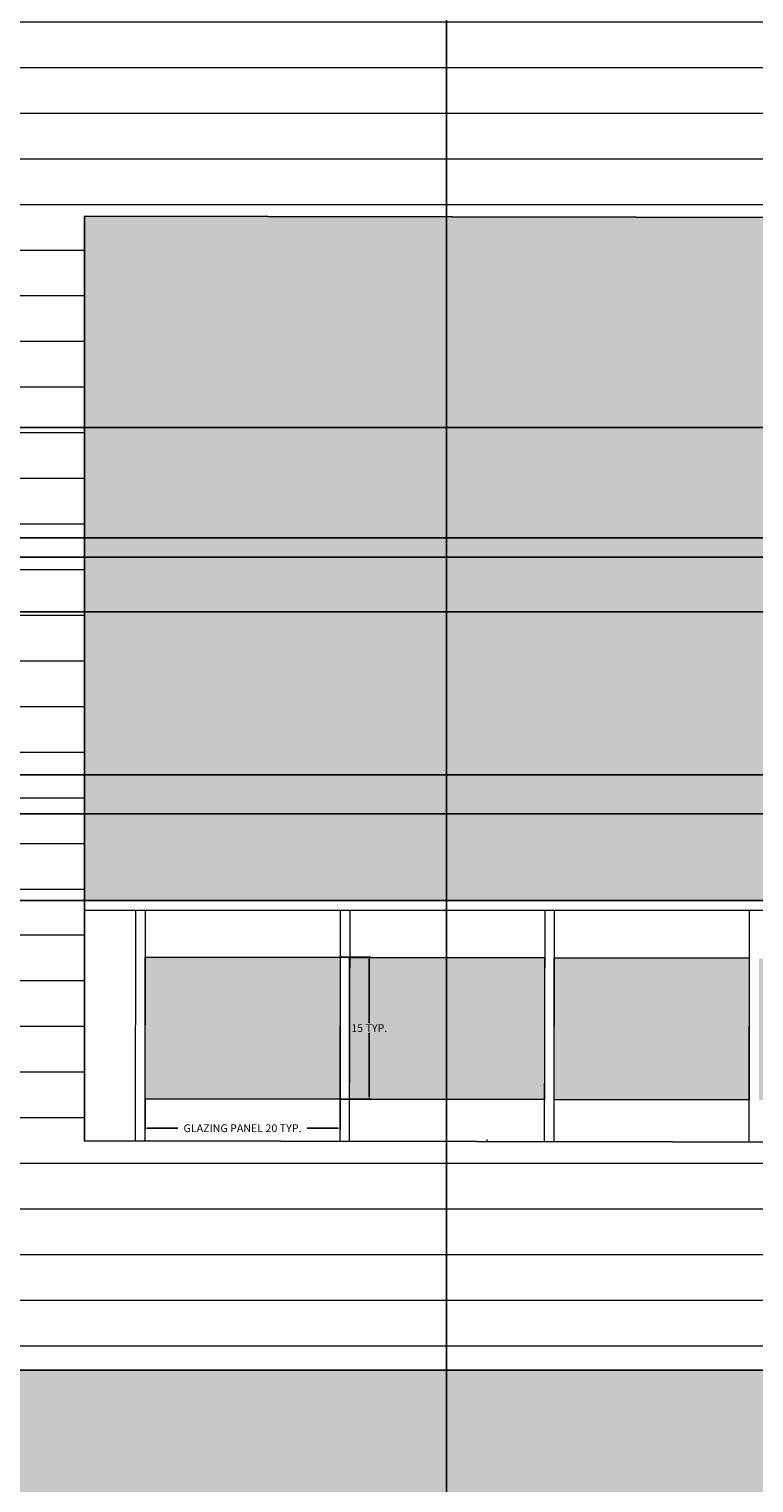
# Model space of a CAD drawing. Units: inches. Extents: x 36 to 594, y 79 to 831.
# Tile 8 of 30: x 113 to 188, y 294 to 446. Entities that reach past the tile are written whole.
import ezdxf

# ---------------------------------------------------------------- set-up
doc = ezdxf.new("R2010")
doc.units = ezdxf.units.IN
doc.header["$MEASUREMENT"] = 0
for name, color, linetype, lineweight in [('A-ANNO-DIMS', 2, 'Continuous', 18), ('A-ELEV', 7, 'Continuous', 25), ('A-ELEV-PATT', 8, 'Continuous', 13), ('A-GLAZ', 4, 'Continuous', 18)]:
    doc.layers.add(name, color=color, linetype=linetype, lineweight=lineweight)
doc.styles.get("Standard").update_dxf_attribs({"font": 'arial.ttf'})
doc.dimstyles.get("Standard").update_dxf_attribs({"dimtxt": 0.8125, "dimasz": 0.18, "dimexe": 0.18, "dimexo": 0.0625, "dimgap": 0.09, "dimtad": 0, "dimtih": 1, "dimtoh": 1, "dimdec": 4, "dimzin": 0, "dimdsep": 46, "dimlunit": 4, "dimtxsty": 'Standard', "dimcen": 0.09, "dimadec": 0, "dimazin": 0, "dimtfac": 1, "dimtdec": 4, "dimtofl": 0, "dimtmove": 0, "dimatfit": 3, "dimfxl": 1, "dimtolj": 1, "dimtzin": 0, "dimarcsym": 0})

# ---------------------------------------------------------------- blocks, each defined once
blk = doc.blocks.new('GLAZ-PANEL')
blk.add_lwpolyline([(0, 14.77), (20.28, 14.77), (20.28, 0), (0, 0)], close=True)
blk = doc.blocks.new('*D3')
at = {"layer": 'A-ANNO-DIMS', "color": 0, "lineweight": -2, "transparency": 16777216}
for p, q in [((125.06, 334.36), (125.06, 331.2)), ((145.34, 334.36), (145.34, 331.2)), ((125.24, 331.38), (128.47, 331.38)), ((145.16, 331.38), (141.93, 331.38))]:
    blk.add_line(p, q, dxfattribs=at)
at = {"layer": 'A-ANNO-DIMS', "color": 0, "transparency": 16777216}
for points in [[(125.24, 331.41), (125.24, 331.35), (125.06, 331.38)], [(145.16, 331.41), (145.16, 331.35), (145.34, 331.38)]]:
    blk.add_solid(points, dxfattribs=at)
at = {"layer": 'Defpoints', "color": 0, "transparency": 16777216}
for p in [(125.06, 334.42), (145.34, 334.42), (145.34, 331.38)]:
    blk.add_point(p, dxfattribs=at)
at = {"layer": 'A-ANNO-DIMS', "color": 0, "transparency": 16777216, "insert": (135.2, 331.38), "char_height": 0.8125, "attachment_point": 5}
blk.add_mtext('\\A1;GLAZING PANEL 20 TYP.', dxfattribs=at)
blk = doc.blocks.new('*D4')
at = {"layer": 'A-ANNO-DIMS', "color": 0, "lineweight": -2, "transparency": 16777216}
for p, q in [((145.4, 349.19), (148.56, 349.19)), ((148.38, 349.01), (148.38, 342.31)), ((148.38, 334.6), (148.38, 341.3)), ((145.4, 334.42), (148.56, 334.42))]:
    blk.add_line(p, q, dxfattribs=at)
at = {"layer": 'A-ANNO-DIMS', "color": 0, "transparency": 16777216}
for points in [[(148.35, 349.01), (148.41, 349.01), (148.38, 349.19)], [(148.35, 334.6), (148.41, 334.6), (148.38, 334.42)]]:
    blk.add_solid(points, dxfattribs=at)
at = {"layer": 'Defpoints', "color": 0, "transparency": 16777216}
for p in [(145.34, 349.19), (148.38, 349.19), (145.34, 334.42)]:
    blk.add_point(p, dxfattribs=at)
at = {"layer": 'A-ANNO-DIMS', "color": 0, "transparency": 16777216, "insert": (148.38, 341.8), "char_height": 0.8125, "attachment_point": 5}
blk.add_mtext('\\A1;15 TYP.', dxfattribs=at)
blk = doc.blocks.new('*D28')
at = {"layer": 'A-ANNO-DIMS', "color": 0, "lineweight": -2, "transparency": 16777216}
for p, q in [((269.3, 796.05), (37.49, 796.05)), ((37.67, 795.87), (37.67, 455.63)), ((37.67, 114.39), (37.67, 454.62)), ((94.8, 114.21), (37.49, 114.21))]:
    blk.add_line(p, q, dxfattribs=at)
at = {"layer": 'A-ANNO-DIMS', "color": 0, "transparency": 16777216}
for points in [[(37.64, 795.87), (37.7, 795.87), (37.67, 796.05)], [(37.64, 114.39), (37.7, 114.39), (37.67, 114.21)]]:
    blk.add_solid(points, dxfattribs=at)
at = {"layer": 'Defpoints', "color": 0, "transparency": 16777216}
for p in [(37.67, 796.05), (269.36, 796.05), (94.87, 114.21)]:
    blk.add_point(p, dxfattribs=at)
at = {"layer": 'A-ANNO-DIMS', "color": 0, "transparency": 16777216, "insert": (37.67, 455.13), "char_height": 0.812, "attachment_point": 5}
blk.add_mtext('\\A1;681.8', dxfattribs=at)
blk = doc.blocks.new('*D60')
at = {"layer": 'A-ANNO-DIMS', "color": 0, "lineweight": -2, "transparency": 16777216}
for p, q in [((103.34, 286.24), (103.34, 830.73)), ((103.52, 830.55), (128.41, 830.55)), ((156.23, 830.55), (131.33, 830.55)), ((156.41, 264.68), (156.41, 830.73))]:
    blk.add_line(p, q, dxfattribs=at)
at = {"layer": 'A-ANNO-DIMS', "color": 0, "transparency": 16777216}
for points in [[(103.52, 830.58), (103.52, 830.52), (103.34, 830.55)], [(156.23, 830.58), (156.23, 830.52), (156.41, 830.55)]]:
    blk.add_solid(points, dxfattribs=at)
at = {"layer": 'Defpoints', "color": 0, "transparency": 16777216}
for p in [(156.41, 830.55), (103.34, 286.18), (156.41, 264.62)]:
    blk.add_point(p, dxfattribs=at)
at = {"layer": 'A-ANNO-DIMS', "color": 0, "transparency": 16777216, "insert": (129.87, 830.55), "char_height": 0.812, "attachment_point": 5}
blk.add_mtext('\\A1;53.07', dxfattribs=at)
blk = doc.blocks.new('*D61')
at = {"layer": 'A-ANNO-DIMS', "color": 0, "lineweight": -2, "transparency": 16777216}
for p, q in [((156.41, 264.68), (156.41, 830.73)), ((156.59, 830.55), (185.26, 830.55)), ((216.85, 830.55), (188.18, 830.55)), ((217.03, 286.24), (217.03, 830.73))]:
    blk.add_line(p, q, dxfattribs=at)
at = {"layer": 'A-ANNO-DIMS', "color": 0, "transparency": 16777216}
for points in [[(156.59, 830.58), (156.59, 830.52), (156.41, 830.55)], [(216.85, 830.58), (216.85, 830.52), (217.03, 830.55)]]:
    blk.add_solid(points, dxfattribs=at)
at = {"layer": 'Defpoints', "color": 0, "transparency": 16777216}
for p in [(217.03, 830.55), (217.03, 286.18), (156.41, 264.62)]:
    blk.add_point(p, dxfattribs=at)
at = {"layer": 'A-ANNO-DIMS', "color": 0, "transparency": 16777216, "insert": (186.72, 830.55), "char_height": 0.812, "attachment_point": 5}
blk.add_mtext('\\A1;60.62', dxfattribs=at)
blk = doc.blocks.new('*D111')
at = {"layer": 'A-ANNO-DIMS', "color": 0, "lineweight": -2, "transparency": 16777216}
for p, q in [((244.76, 364.09), (37.49, 364.09)), ((37.67, 363.91), (37.67, 360.09)), ((37.67, 355.26), (37.67, 359.08)), ((241.29, 355.08), (37.49, 355.08))]:
    blk.add_line(p, q, dxfattribs=at)
at = {"layer": 'A-ANNO-DIMS', "color": 0, "transparency": 16777216}
for points in [[(37.64, 363.91), (37.7, 363.91), (37.67, 364.09)], [(37.64, 355.26), (37.7, 355.26), (37.67, 355.08)]]:
    blk.add_solid(points, dxfattribs=at)
at = {"layer": 'Defpoints', "color": 0, "transparency": 16777216}
for p in [(37.67, 364.09), (244.82, 364.09), (241.36, 355.08)]:
    blk.add_point(p, dxfattribs=at)
at = {"layer": 'A-ANNO-DIMS', "color": 0, "transparency": 16777216, "insert": (37.67, 359.59), "char_height": 0.812, "attachment_point": 5}
blk.add_mtext('\\A1;9.005', dxfattribs=at)
blk = doc.blocks.new('*D112')
at = {"layer": 'A-ANNO-DIMS', "color": 0, "lineweight": -2, "transparency": 16777216}
for p, q in [((244.76, 368.16), (37.49, 368.16)), ((37.67, 367.98), (37.67, 366.63)), ((37.67, 364.27), (37.67, 365.62)), ((244.76, 364.09), (37.49, 364.09))]:
    blk.add_line(p, q, dxfattribs=at)
at = {"layer": 'A-ANNO-DIMS', "color": 0, "transparency": 16777216}
for points in [[(37.64, 367.98), (37.7, 367.98), (37.67, 368.16)], [(37.64, 364.27), (37.7, 364.27), (37.67, 364.09)]]:
    blk.add_solid(points, dxfattribs=at)
at = {"layer": 'Defpoints', "color": 0, "transparency": 16777216}
for p in [(37.67, 368.16), (244.82, 368.16), (244.82, 364.09)]:
    blk.add_point(p, dxfattribs=at)
at = {"layer": 'A-ANNO-DIMS', "color": 0, "transparency": 16777216, "insert": (37.67, 366.13), "char_height": 0.812, "attachment_point": 5}
blk.add_mtext('\\A1;4.074', dxfattribs=at)
blk = doc.blocks.new('*D113')
at = {"layer": 'A-ANNO-DIMS', "color": 0, "lineweight": -2, "transparency": 16777216}
for p, q in [((244.76, 385.12), (37.49, 385.12)), ((37.67, 384.94), (37.67, 377.15)), ((37.67, 368.34), (37.67, 376.14)), ((244.76, 368.16), (37.49, 368.16))]:
    blk.add_line(p, q, dxfattribs=at)
at = {"layer": 'A-ANNO-DIMS', "color": 0, "transparency": 16777216}
for points in [[(37.64, 384.94), (37.7, 384.94), (37.67, 385.12)], [(37.64, 368.34), (37.7, 368.34), (37.67, 368.16)]]:
    blk.add_solid(points, dxfattribs=at)
at = {"layer": 'Defpoints', "color": 0, "transparency": 16777216}
for p in [(37.67, 385.12), (244.82, 385.12), (244.82, 368.16)]:
    blk.add_point(p, dxfattribs=at)
at = {"layer": 'A-ANNO-DIMS', "color": 0, "transparency": 16777216, "insert": (37.67, 376.64), "char_height": 0.812, "attachment_point": 5}
blk.add_mtext('\\A1;16.957', dxfattribs=at)
blk = doc.blocks.new('*D114')
at = {"layer": 'A-ANNO-DIMS', "color": 0, "lineweight": -2, "transparency": 16777216}
for p, q in [((241.29, 390.79), (37.49, 390.79)), ((37.67, 390.61), (37.67, 388.46)), ((37.67, 385.3), (37.67, 387.45)), ((244.76, 385.12), (37.49, 385.12))]:
    blk.add_line(p, q, dxfattribs=at)
at = {"layer": 'A-ANNO-DIMS', "color": 0, "transparency": 16777216}
for points in [[(37.64, 390.61), (37.7, 390.61), (37.67, 390.79)], [(37.64, 385.3), (37.7, 385.3), (37.67, 385.12)]]:
    blk.add_solid(points, dxfattribs=at)
at = {"layer": 'Defpoints', "color": 0, "transparency": 16777216}
for p in [(37.67, 390.79), (241.36, 390.79), (244.82, 385.12)]:
    blk.add_point(p, dxfattribs=at)
at = {"layer": 'A-ANNO-DIMS', "color": 0, "transparency": 16777216, "insert": (37.67, 387.96), "char_height": 0.812, "attachment_point": 5}
blk.add_mtext('\\A1;5.672', dxfattribs=at)
blk = doc.blocks.new('*D115')
at = {"layer": 'A-ANNO-DIMS', "color": 0, "lineweight": -2, "transparency": 16777216}
for p, q in [((241.29, 392.79), (37.49, 392.79)), ((37.67, 392.61), (37.67, 392.29)), ((241.29, 390.79), (37.49, 390.79)), ((37.67, 390.97), (37.67, 391.29))]:
    blk.add_line(p, q, dxfattribs=at)
at = {"layer": 'A-ANNO-DIMS', "color": 0, "transparency": 16777216}
for points in [[(37.64, 392.61), (37.7, 392.61), (37.67, 392.79)], [(37.64, 390.97), (37.7, 390.97), (37.67, 390.79)]]:
    blk.add_solid(points, dxfattribs=at)
at = {"layer": 'Defpoints', "color": 0, "transparency": 16777216}
for p in [(37.67, 392.79), (241.36, 392.79), (241.36, 390.79)]:
    blk.add_point(p, dxfattribs=at)
at = {"layer": 'A-ANNO-DIMS', "color": 0, "transparency": 16777216, "insert": (37.67, 391.79), "char_height": 0.812, "attachment_point": 5}
blk.add_mtext('\\A1;2', dxfattribs=at)
blk = doc.blocks.new('*D116')
at = {"layer": 'A-ANNO-DIMS', "color": 0, "lineweight": -2, "transparency": 16777216}
for p, q in [((241.29, 404.27), (37.49, 404.27)), ((37.67, 404.09), (37.67, 399.04)), ((37.67, 392.97), (37.67, 398.03)), ((241.29, 392.79), (37.49, 392.79))]:
    blk.add_line(p, q, dxfattribs=at)
at = {"layer": 'A-ANNO-DIMS', "color": 0, "transparency": 16777216}
for points in [[(37.64, 404.09), (37.7, 404.09), (37.67, 404.27)], [(37.64, 392.97), (37.7, 392.97), (37.67, 392.79)]]:
    blk.add_solid(points, dxfattribs=at)
at = {"layer": 'Defpoints', "color": 0, "transparency": 16777216}
for p in [(37.67, 404.27), (241.36, 404.27), (241.36, 392.79)]:
    blk.add_point(p, dxfattribs=at)
at = {"layer": 'A-ANNO-DIMS', "color": 0, "transparency": 16777216, "insert": (37.67, 398.53), "char_height": 0.812, "attachment_point": 5}
blk.add_mtext('\\A1;11.481', dxfattribs=at)

msp = doc.modelspace()

# ---------------------------------------------------------------- hatches: boundary and pattern name
at = {"layer": 'A-ELEV-PATT'}
h = msp.add_hatch(color=256, dxfattribs=at)
h.dxf.hatch_style = 1
h.paths.add_polyline_path([(398.0873, 796.0465), (269.3592, 796.0465), (269.3592, 770.1455), (397.8159, 770.1455)])
h.paths.add_polyline_path([(397.7518, 764.0341), (269.3592, 764.0341), (269.3592, 630.0394), (341.8367, 630.0394), (341.8367, 720.595), (335.0881, 728.3699), (329.982, 735.3373), (345.3661, 727.7743), (397.1052, 702.3389)])
h.paths.add_polyline_path([(341.8367, 594.2124), (201.4189, 594.2124), (201.4189, 475.4136), (232.8216, 475.4136), (232.8216, 524.6037), (341.8367, 524.6037)])
h.paths.add_polyline_path([(177.525, 594.2124), (118.7598, 594.2124), (118.7598, 450.2124), (177.525, 450.2124)])
h.paths.add_polyline_path([(424.4958, 594.2124), (365.7306, 594.2124), (365.7306, 450.2124), (424.4958, 450.2124)])
h.paths.add_polyline_path([(241.3553, 404.2737), (355.8569, 404.2737), (355.8569, 355.0836), (424.5492, 355.0836), (424.5492, 425.7333), (118.7598, 426.2844), (118.7598, 355.0836), (241.3553, 355.0836)])
h.paths.add_polyline_path([(448.3898, 306.2124), (217.0273, 306.2124), (217.0273, 142.2124), (254.0293, 142.2124), (254.0293, 150.9347), (254.0293, 286.1802), (401.5491, 286.1802), (401.5491, 150.9347), (401.5491, 142.2124), (448.3898, 142.2124)])
h.paths.add_polyline_path([(448.3898, 142.2124), (401.5491, 142.2124), (217.0273, 142.2124), (217.0273, 114.2124), (448.3898, 114.2124)])
h.paths.add_polyline_path([(217.0273, 306.2124), (174.7353, 306.2124), (94.8658, 306.2124), (94.8658, 162.2124), (103.3368, 162.2124), (103.3368, 264.6224), (103.3368, 286.1802), (217.0273, 286.1802)])
h = msp.add_hatch(color=256, dxfattribs=at)
h.dxf.hatch_style = 1
h.set_gradient(color1=(192, 192, 192), color2=(0, 0, 0))
h.paths.add_polyline_path([(243.19, 469.3251), (222.9132, 469.3251), (222.9132, 454.5571), (243.1634, 454.5571)])
h.paths.add_polyline_path([(264.4667, 469.2868), (244.1899, 469.2868), (244.1899, 454.5188), (264.4401, 454.5188)])
h.paths.add_polyline_path([(285.7435, 469.2484), (265.4667, 469.2484), (265.4667, 454.4804), (285.7168, 454.4804)])
h.paths.add_polyline_path([(307.0202, 469.2101), (286.7434, 469.2101), (286.7434, 454.4421), (306.9936, 454.4421)])
h.paths.add_polyline_path([(328.2969, 469.1717), (308.0201, 469.1717), (308.0201, 454.4037), (328.2703, 454.4037)])
h.paths.add_polyline_path([(341.8367, 469.1334), (329.2969, 469.1334), (329.2969, 454.3654), (341.8367, 454.3654)])
h.paths.add_polyline_path([(221.9133, 469.3635), (201.6365, 469.3635), (201.6365, 454.5955), (221.8866, 454.5955)])
h.paths.add_polyline_path([(145.3401, 349.1868), (125.0633, 349.1868), (125.0633, 334.4189), (145.3134, 334.4189)])
h.paths.add_polyline_path([(166.6168, 349.1485), (146.34, 349.1485), (146.34, 334.3805), (166.5902, 334.3805)])
h.paths.add_polyline_path([(187.8935, 349.1101), (167.6167, 349.1101), (167.6167, 334.3422), (187.8669, 334.3422)])
h.paths.add_polyline_path([(209.1703, 349.0718), (188.8935, 349.0718), (188.8935, 334.3038), (209.1436, 334.3038)])
h.paths.add_polyline_path([(230.447, 349.0335), (210.1702, 349.0335), (210.1702, 334.2655), (230.4204, 334.2655)])
h.paths.add_polyline_path([(251.7237, 348.9951), (231.4469, 348.9951), (231.4469, 334.2271), (251.6971, 334.2271)])
h.paths.add_polyline_path([(273.0005, 348.9568), (252.7236, 348.9568), (252.7236, 334.1888), (272.9738, 334.1888)])
h.paths.add_polyline_path([(294.2772, 348.9184), (274.0004, 348.9184), (274.0004, 334.1504), (294.2506, 334.1504)])
h.paths.add_polyline_path([(315.5539, 348.8801), (295.2771, 348.8801), (295.2771, 334.1121), (315.5273, 334.1121)])
h.paths.add_polyline_path([(336.8306, 348.8417), (316.5538, 348.8417), (316.5538, 334.0737), (336.804, 334.0737)])
h.paths.add_polyline_path([(358.1074, 348.8034), (337.8306, 348.8034), (337.8306, 334.0354), (358.0808, 334.0354)])
h.paths.add_polyline_path([(379.3841, 348.765), (359.1073, 348.765), (359.1073, 333.997), (379.3575, 333.997)])
h.paths.add_polyline_path([(400.6608, 348.7267), (380.384, 348.7267), (380.384, 333.9587), (400.6342, 333.9587)])
h.paths.add_polyline_path([(421.9376, 348.6883), (401.6608, 348.6883), (401.6608, 333.9204), (421.911, 333.9204)])
h.paths.add_polyline_path([(103.3368, 162.2124), (94.8658, 162.2124), (94.8658, 150.2124), (94.8658, 114.2124), (103.3368, 114.2124)])
h.paths.add_polyline_path([(217.0273, 132.2124), (103.3368, 132.2124), (103.3368, 122.2124), (217.0273, 122.2124)])
h.paths.add_polyline_path([(217.0273, 122.2124), (103.3368, 122.2124), (103.3368, 114.2124), (217.0273, 114.2124)])
h.paths.add_polyline_path([(217.0273, 142.2124), (174.7353, 142.2124), (103.3368, 142.2124), (103.3368, 132.2124), (217.0273, 132.2124)])
h.paths.add_polyline_path([(217.0273, 152.2124), (103.3368, 152.2124), (103.3368, 142.2124), (174.7353, 142.2124), (217.0273, 142.2124)])
h.paths.add_polyline_path([(217.0273, 162.2124), (103.3368, 162.2124), (103.3368, 152.2124), (217.0273, 152.2124)])
h = msp.add_hatch(dxfattribs=at)
h.set_pattern_fill('ANSI31', color=256, scale=38, angle=135)
h.paths.add_polyline_path([(448.3898, 450.2124), (94.8658, 450.2124), (94.8658, 306.2124), (174.7353, 306.2124), (448.3898, 306.2124), (448.3898, 367.5118)])
h.paths.add_polyline_path([(424.5492, 425.7333), (424.5492, 329.5325), (118.7598, 330.0836), (118.7598, 354.0836), (118.7598, 426.2844)], flags=16)
h.paths.add_polyline_path([(355.8569, 404.2737), (355.8569, 355.0836), (241.3553, 355.0836), (241.3553, 404.2737)], flags=0)
h.paths.add_polyline_path([(269.0393, 390.7924), (269.0393, 355.0836), (244.8248, 355.0836), (244.8248, 364.0887), (263.8892, 364.0887), (263.8892, 355.0836), (267.0393, 355.0836), (267.0393, 390.7924)], flags=0)
h.paths.add_polyline_path([(303.9765, 436.9126, -1), (313.1496, 436.9126, -1)], flags=16)
h.paths.add_polyline_path([(421.9473, 354.0836), (421.9376, 348.6883), (421.9376, 333.9204), (401.6342, 333.9204), (401.6705, 354.0836), (400.6705, 354.0836), (400.6608, 348.7267), (400.6608, 333.9587), (380.3574, 333.9587), (380.3937, 354.0836), (379.3937, 354.0836), (379.3841, 348.765), (379.3841, 333.997), (359.0807, 333.997), (359.1169, 354.0836), (358.1169, 354.0836), (358.1074, 348.8034), (358.1074, 334.0354), (337.804, 334.0354), (337.8401, 354.0836), (336.8401, 354.0836), (336.8306, 348.8417), (336.8306, 334.0737), (316.5272, 334.0737), (316.5633, 354.0836), (315.5633, 354.0836), (315.5539, 348.8801), (315.5539, 334.1121), (295.2505, 334.1121), (295.2865, 354.0836), (294.2865, 354.0836), (294.2772, 348.9184), (294.2772, 334.1504), (273.9738, 334.1504), (274.0097, 354.0836), (273.0097, 354.0836), (273.0005, 348.9568), (273.0005, 334.1888), (252.697, 334.1888), (252.7329, 354.0836), (251.7329, 354.0836), (251.7237, 348.9951), (251.7237, 334.2271), (231.4203, 334.2271), (231.4561, 354.0836), (230.4561, 354.0836), (230.447, 349.0335), (230.447, 334.2655), (210.1436, 334.2655), (210.1793, 354.0836), (209.1793, 354.0836), (209.1703, 349.0718), (209.1703, 334.3038), (188.8668, 334.3038), (188.9025, 354.0836), (187.9025, 354.0836), (187.8935, 349.1101), (187.8935, 334.3422), (167.5901, 334.3422), (167.6257, 354.0836), (166.6257, 354.0836), (166.6168, 349.1485), (166.6168, 334.3805), (146.3134, 334.3805), (146.3489, 354.0836), (145.3489, 354.0836), (145.3401, 349.1868), (145.3401, 334.4189), (125.0366, 334.4189), (125.0721, 354.0836)], flags=0)
h.paths.add_polyline_path([(266.285, 436.9126, -1), (275.458, 436.9126, -1)], flags=16)
h.paths.add_polyline_path([(367.0204, 316.8739, -1), (357.8474, 316.8739, -1)], flags=16)
h.paths.add_polyline_path([(347.6933, 316.8739, -1), (338.5202, 316.8739, -1)], flags=16)
h.paths.add_polyline_path([(329.574, 316.8739, -1), (320.401, 316.8739, -1)], flags=16)
h.paths.add_polyline_path([(263.8892, 385.1199), (263.8892, 368.1628), (244.8248, 368.1628), (244.8248, 385.1199)], flags=0)
h.paths.add_polyline_path([(216.2543, 436.9126, -1), (225.4274, 436.9126, -1)], flags=16)
h.paths.add_polyline_path([(275.458, 316.8739, -1), (266.285, 316.8739, -1)], flags=16)
h.paths.add_polyline_path([(225.4274, 316.8739, -1), (216.2543, 316.8739, -1)], flags=16)

# ---------------------------------------------------------------- linework, layer by layer
at = {"layer": 'A-ELEV'}
for p, q in [((94.8658, 306.2124), (174.7353, 306.2124)), ((174.7353, 306.2124), (448.3898, 306.2124))]:
    msp.add_line(p, q, dxfattribs=at)
msp.add_lwpolyline([(118.7598, 426.2844), (424.5492, 425.7333), (424.5492, 329.5325), (118.7598, 330.0836)], close=True, dxfattribs=at)
at = {"layer": 'A-GLAZ'}
for p, q in [((156.5389, 426.2163), (156.5389, 426.2124)), ((118.7598, 378.2124), (118.8525, 378.2124)), ((118.7598, 355.0836), (424.5492, 355.0836)), ((118.7598, 330.0836), (118.7598, 354.0836)), ((118.7598, 354.0836), (424.5492, 354.0836)), ((124.0721, 354.0836), (124.0288, 330.0741)), ((125.0721, 354.0818), (125.0288, 330.0723)), ((145.3489, 354.0836), (145.3056, 330.0741)), ((146.3489, 354.0818), (146.3056, 330.0723)), ((166.6257, 354.0836), (166.5823, 330.0357)), ((167.6257, 354.0836), (167.5823, 330.0339)), ((187.9025, 354.0836), (187.8591, 329.9974)), ((160.6519, 330.0081), (160.6519, 330.2124))]:
    msp.add_line(p, q, dxfattribs=at)

# ---------------------------------------------------------------- block references
for p in [(125.063, 334.419), (146.3397, 334.3807), (167.6165, 334.3423)]:
    msp.add_blockref('GLAZ-PANEL', p, dxfattribs=at)

# ---------------------------------------------------------------- dimensions: what is measured, and where the dimension line sits
at = {"layer": 'A-ANNO-DIMS'}
for base, p1, p2, picture, middle in [((156.4069, 830.5465), (103.3368, 286.1802), (156.4069, 264.6224), '*D60', (129.8718, 830.5465)), ((217.0273, 830.5465), (156.4069, 264.6224), (217.0273, 286.1802), '*D61', (186.7171, 830.5465))]:
    dim = msp.add_linear_dim(base=base, p1=p1, p2=p2, dimstyle='Standard', override={"dimdec": 2, "dimlfac": 1, "dimrnd": 0, "dimzin": 0, "dimdsep": 46, "dimlunit": 2}, dxfattribs=at)
    dim.commit()
    dim.dimension.update_dxf_attribs({"geometry": picture, "text_midpoint": middle})
for base, p1, p2, override, picture, middle in [((37.6733, 796.0465), (94.8658, 114.2124), (269.3592, 796.0465), {"dimdec": 1, "dimlfac": 1, "dimrnd": 0, "dimzin": 0, "dimdsep": 46, "dimlunit": 2}, '*D28', (37.6733, 455.1294)), ((37.6733, 404.2737), (241.3553, 392.7924), (241.3553, 404.2737), {"dimdec": 3, "dimlfac": 1, "dimrnd": 0, "dimzin": 0, "dimdsep": 46, "dimlunit": 2}, '*D116', (37.6733, 398.533)), ((37.6733, 392.7924), (241.3553, 390.7924), (241.3553, 392.7924), {"dimdec": 0, "dimlfac": 1, "dimrnd": 0, "dimzin": 0, "dimdsep": 46, "dimlunit": 2}, '*D115', (37.6733, 391.7924)), ((37.67335, 390.79236), (244.82478, 385.11988), (241.3553, 390.79236), {"dimdec": 3, "dimlfac": 1, "dimrnd": 0, "dimzin": 0, "dimdsep": 46, "dimlunit": 2}, '*D114', (37.67335, 387.95612)), ((37.6733, 385.1199), (244.8248, 368.1628), (244.8248, 385.1199), {"dimdec": 3, "dimlfac": 1, "dimrnd": 0, "dimzin": 0, "dimdsep": 46, "dimlunit": 2}, '*D113', (37.6733, 376.6414)), ((37.6733, 368.1628), (244.8248, 364.0887), (244.8248, 368.1628), {"dimdec": 3, "dimlfac": 1, "dimrnd": 0, "dimzin": 0, "dimdsep": 46, "dimlunit": 2}, '*D112', (37.6733, 366.1258)), ((37.6733, 364.0887), (241.3553, 355.0836), (244.8248, 364.0887), {"dimdec": 3, "dimlfac": 1, "dimrnd": 0, "dimzin": 0, "dimdsep": 46, "dimlunit": 2}, '*D111', (37.6733, 359.5862))]:
    dim = msp.add_linear_dim(base=base, p1=p1, p2=p2, angle=90, dimstyle='Standard', override=override, dxfattribs=at)
    dim.commit()
    dim.dimension.update_dxf_attribs({"geometry": picture, "text_midpoint": middle})
dim = msp.add_linear_dim(base=(148.3816, 349.1868), p1=(145.3401, 334.4189), p2=(145.3401, 349.1868), angle=90, text='<> TYP.', dimstyle='Standard', override={"dimdec": 0, "dimlfac": 1, "dimrnd": 0, "dimzin": 0, "dimdsep": 46, "dimlunit": 2}, dxfattribs=at)
dim.commit()
dim.dimension.update_dxf_attribs({"geometry": '*D4', "text_midpoint": (148.3816, 341.8029)})
dim = msp.add_linear_dim(base=(145.3401, 331.3773), p1=(125.0633, 334.4189), p2=(145.3401, 334.4189), text='GLAZING PANEL <> TYP.', dimstyle='Standard', override={"dimdec": 0, "dimlfac": 1, "dimrnd": 0, "dimzin": 0, "dimdsep": 46, "dimlunit": 2}, dxfattribs=at)
dim.commit()
dim.dimension.update_dxf_attribs({"geometry": '*D3', "text_midpoint": (135.2017, 331.3773)})

doc.saveas('drawing.dxf')
